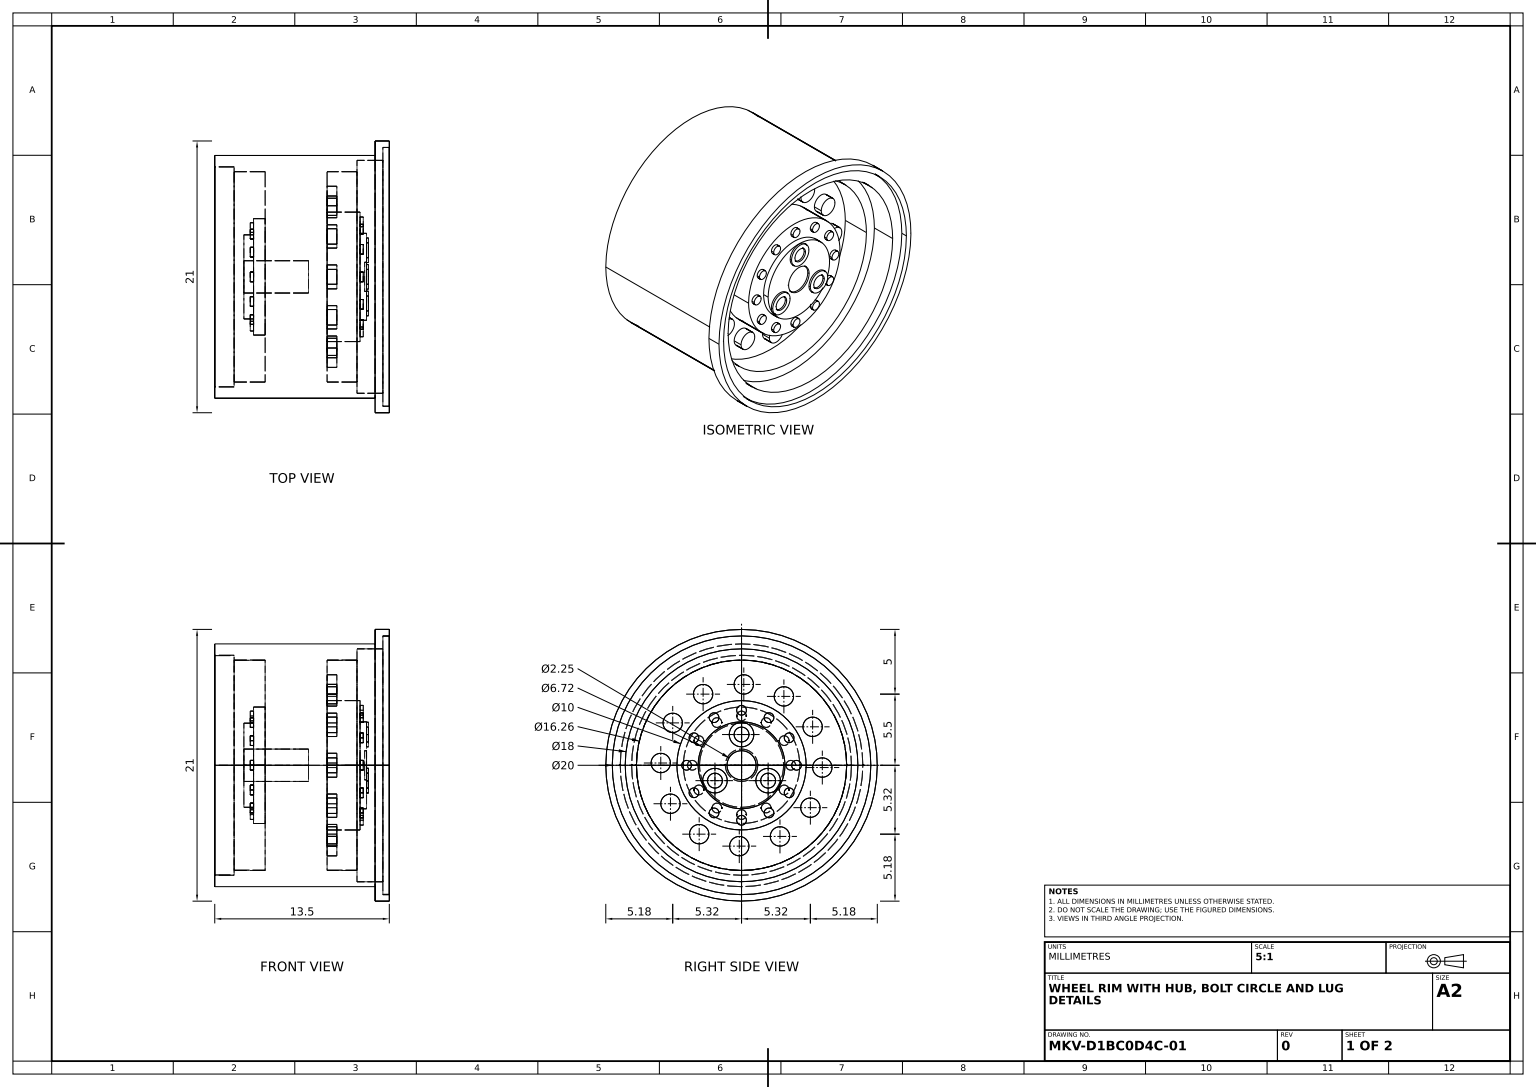
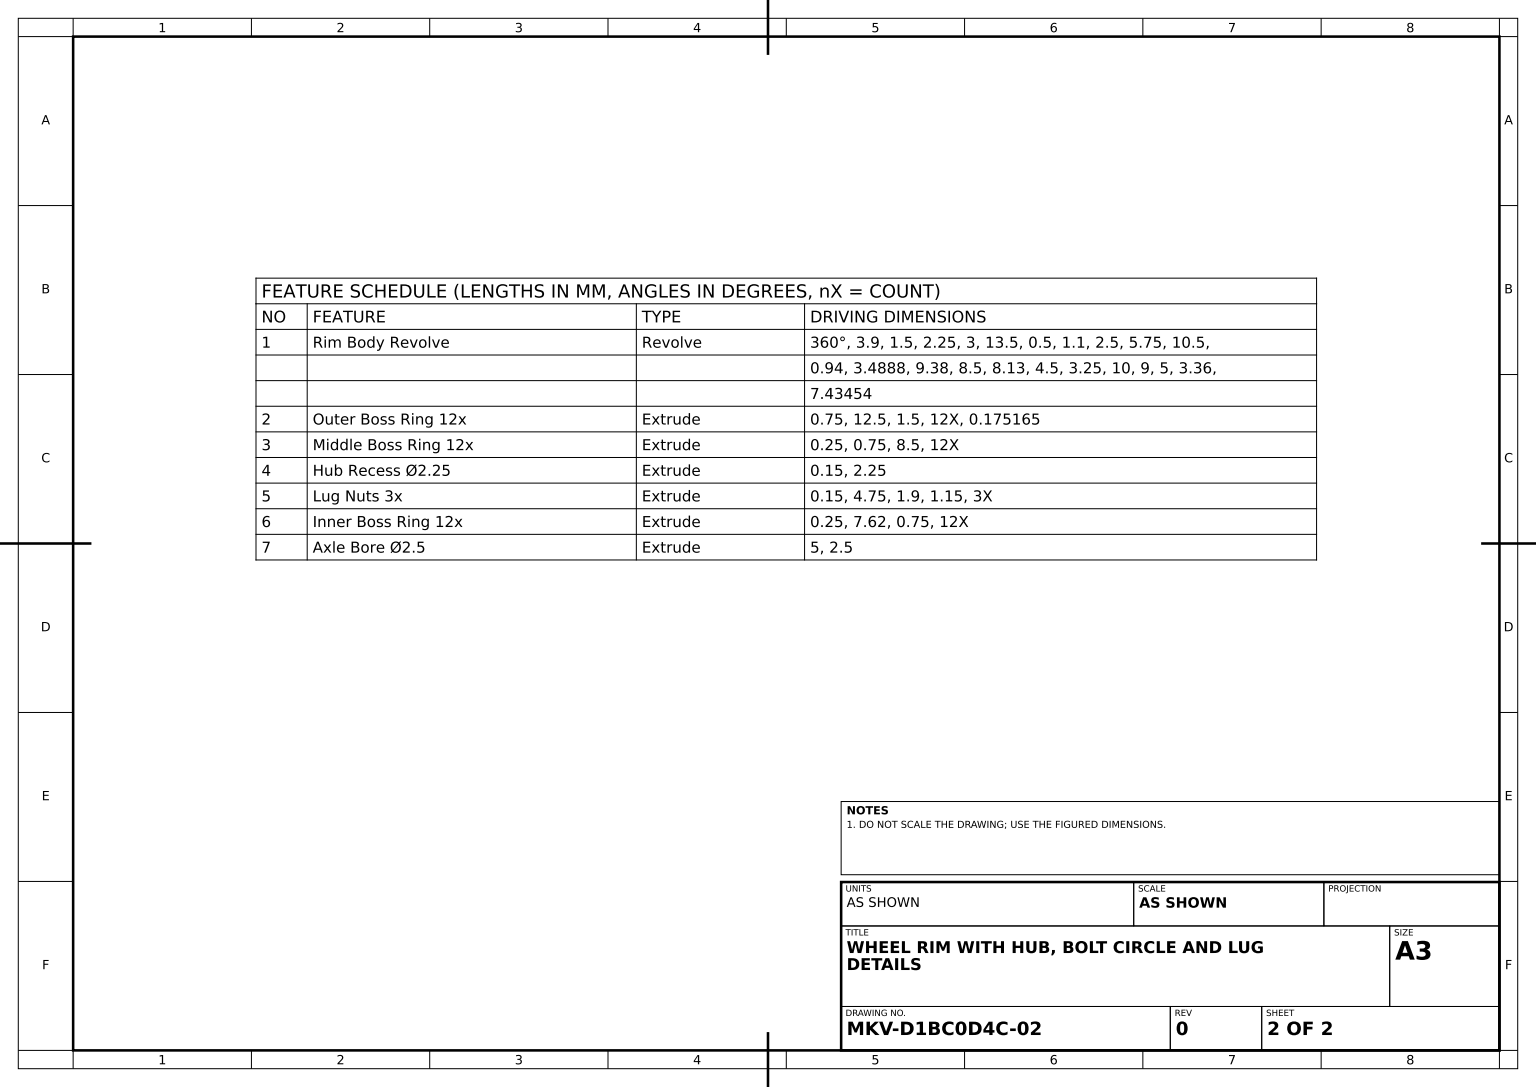
SolidWorks part; units mm, degrees
material "Plain Carbon Steel"
ref_plane "Front Plane" through (0, 0, 0) normal (0, 0, 1) x (1, 0, 0)
ref_plane "Top Plane" through (0, 0, 0) normal (0, 1, 0) x (1, 0, 0)
ref_plane "Right Plane" through (0, 0, 0) normal (1, 0, 0) x (0, 0, -1)
sketch "Rim Profile Sketch" plane through (0, 0, 0) normal (0, 0, 1) x (1, 0, 0)
  line L0 (0, 9.38) -> (0, 0) construction
  line L1 (0, 0) -> (9.8961, 0) construction
  line L2 (0, 9.38) -> (-7.75, 9.38)
  line L3 (-7.75, 9.38) -> (-7.75, 8.5)
  line L4 (-7.75, 8.5) -> (-6.25, 8.5)
  line L5 (-6.25, 8.5) -> (-6.25, 8.13)
  line L6 (-6.25, 8.13) -> (-3.85, 8.13)
  line L7 (-3.85, 8.13) -> (-3.85, 4.5)
  line L8 (-3.85, 4.5) -> (-4.75, 4.5)
  line L9 (-4.75, 4.5) -> (-4.75, 3.25)
  line L10 (-4.75, 3.25) -> (-5.5, 3.25)
  line L11 (-5.5, 3.25) -> (-5.5, 0)
  line L12 (-5.5, 0) -> (7.4345, 0)
  line L13 (0, 9.38) -> (4.65, 9.38)
  line L14 (4.65, 9.38) -> (4.65, 10.5)
  line L15 (4.65, 10.5) -> (5.75, 10.5)
  line L16 (5.75, 10.5) -> (5.75, 10)
  line L17 (5.75, 10) -> (5.25, 10)
  line L18 (5.25, 10) -> (5.25, 9)
  line L19 (5.25, 9) -> (3.25, 9)
  line L20 (3.25, 9) -> (3.25, 8.13)
  line L21 (3.25, 8.13) -> (0.94, 8.13)
  line L22 (0.94, 8.13) -> (0.94, 5)
  line L23 (0.94, 5) -> (3.4888, 5)
  line L24 (3.4888, 5) -> (3.4888, 3.36)
  line L25 (3.4888, 3.36) -> (3.9888, 3.36)
  line L26 (3.9888, 3.36) -> (3.9888, 0)
  point P36 (5.75, 10.25)
  dimension "D1" = 9.38
  dimension "D2" = 8.5
  dimension "D3" = 8.13
  dimension "D4" = 4.5
  dimension "D5" = 3.25
  dimension "D6" = 3.9
  dimension "D7" = 1.5
  dimension "D8" = 2.25
  dimension "D9" = 3
  dimension "D10" = 13.5
  dimension "D11" = 0.5
  dimension "D12" = 1.1
  dimension "D13" = 2.5
  dimension "D14" = 5.75
  dimension "D15" = 0.5
  dimension "D16" = 10.5
  dimension "D17" = 10
  dimension "D18" = 9
  dimension "D19" = 8.13
  dimension "D20" = 5
  dimension "D21" = 3.36
  dimension "D22" = 0.94
  dimension "D23" = 3.4888
  dimension "D24" = 7.4345
revolve "Rim Body Revolve" add sketch "Rim Profile Sketch" angle 360 about L1
sketch "Outer Boss Ring Sketch 12xØ1.5" plane through (0.94, 0, 0) normal (1, 0, 0) x (0, 0, -1)
  circle A0 centre (0, 0) radius 6.25 construction
  circle A1 centre (0.1752, 6.2475) radius 0.75
  circle A2 centre (3.2755, 5.323) radius 0.75
  circle A3 centre (5.4981, 2.9721) radius 0.75
  circle A4 centre (6.2475, -0.1752) radius 0.75
  circle A5 centre (5.323, -3.2755) radius 0.75
  circle A6 centre (2.9721, -5.4981) radius 0.75
  circle A7 centre (-0.1752, -6.2475) radius 0.75
  circle A8 centre (-3.2755, -5.323) radius 0.75
  circle A9 centre (-5.4981, -2.9721) radius 0.75
  circle A10 centre (-6.2475, 0.1752) radius 0.75
  circle A11 centre (-5.323, 3.2755) radius 0.75
  circle A12 centre (-2.9721, 5.4981) radius 0.75
  circle A13 centre (0, 0) radius 5 construction
  point P29 (0, 0)
  dimension "D1" = 12.5
  dimension "D2" = 1.5
  dimension "D4" = 0.1752
  dimension "D3" = 12
extrude "Outer Boss Ring 12x" add sketch "Outer Boss Ring Sketch 12xØ1.5" along normal blind 0.75
sketch "Middle Boss Ring Sketch 12x" plane through (3.4888, 0, 0) normal (1, 0, 0) x (0, 0, -1)
  circle A0 centre (0, 0) radius 4.25 construction
  circle A1 centre (0, 4.25) radius 0.375
  circle A2 centre (2.125, 3.6806) radius 0.375
  circle A3 centre (3.6806, 2.125) radius 0.375
  circle A4 centre (4.25, 0) radius 0.375
  circle A5 centre (3.6806, -2.125) radius 0.375
  circle A6 centre (2.125, -3.6806) radius 0.375
  circle A7 centre (0, -4.25) radius 0.375
  circle A8 centre (-2.125, -3.6806) radius 0.375
  circle A9 centre (-3.6806, -2.125) radius 0.375
  circle A10 centre (-4.25, 0) radius 0.375
  circle A11 centre (-3.6806, 2.125) radius 0.375
  circle A12 centre (-2.125, 3.6806) radius 0.375
  point P30 (0, 0)
  dimension "D1" = 0.75
  dimension "D2" = 8.5
  dimension "D3" = 12
extrude "Middle Boss Ring 12x" add sketch "Middle Boss Ring Sketch 12x" along normal blind 0.25
sketch "Hub Recess Sketch Ø2.25" plane through (3.9888, 0, 0) normal (1, 0, 0) x (0, 0, -1)
  circle A0 centre (0, 0) radius 1.125
  dimension "D1" = 2.25
extrude "Hub Recess Ø2.25" cut sketch "Hub Recess Sketch Ø2.25" against normal blind 0.15
sketch "Lug Nuts Sketch 3x" plane through (3.9888, 0, 0) normal (1, 0, 0) x (0, 0, -1)
  circle A0 centre (0, 0) radius 2.375 construction
  circle A1 centre (0, 2.375) radius 0.95
  circle A2 centre (0, 2.375) radius 0.575
  circle A3 centre (2.0568, -1.1875) radius 0.95
  circle A4 centre (2.0568, -1.1875) radius 0.575
  circle A5 centre (-2.0568, -1.1875) radius 0.95
  circle A6 centre (-2.0568, -1.1875) radius 0.575
  point P14 (0, 0)
  dimension "D1" = 4.75
  dimension "D2" = 1.9
  dimension "D3" = 1.15
  dimension "D4" = 3
extrude "Lug Nuts 3x" add sketch "Lug Nuts Sketch 3x" along normal blind 0.15
sketch "Inner Boss Ring Sketch 12x" plane through (-4.75, 0, 0) normal (-1, 0, 0) x (0, 0, 1)
  circle A0 centre (0, 0) radius 3.81 construction
  circle A1 centre (0, 3.81) radius 0.375
  circle A2 centre (1.905, 3.2996) radius 0.375
  circle A3 centre (3.2996, 1.905) radius 0.375
  circle A4 centre (3.81, 0) radius 0.375
  circle A5 centre (3.2996, -1.905) radius 0.375
  circle A6 centre (1.905, -3.2996) radius 0.375
  circle A7 centre (0, -3.81) radius 0.375
  circle A8 centre (-1.905, -3.2996) radius 0.375
  circle A9 centre (-3.2996, -1.905) radius 0.375
  circle A10 centre (-3.81, 0) radius 0.375
  circle A11 centre (-3.2996, 1.905) radius 0.375
  circle A12 centre (-1.905, 3.2996) radius 0.375
  point P30 (0, 0)
  dimension "D1" = 7.62
  dimension "D2" = 0.75
  dimension "D3" = 12
extrude "Inner Boss Ring 12x" add sketch "Inner Boss Ring Sketch 12x" along normal blind 0.25
sketch "Axle Bore Sketch Ø2.5" plane through (-5.5, 0, 0) normal (-1, 0, 0) x (0, 0, 1)
  circle A0 centre (0, 0) radius 1.25
  dimension "D1" = 2.5
extrude "Axle Bore Ø2.5" cut sketch "Axle Bore Sketch Ø2.5" against normal blind 5
